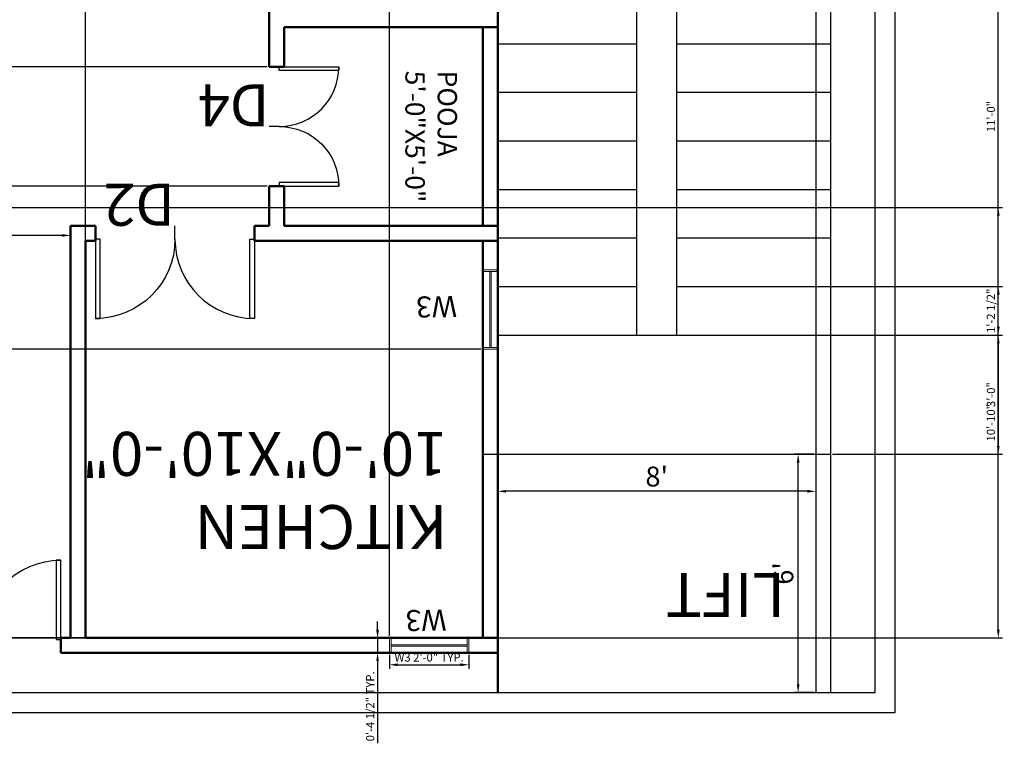
# Model space of a CAD drawing. Units: inches. Extents: x 1989 to 2637, y 1032 to 1611.
# Tile 3 of 5: x 2340 to 2637, y 1056 to 1274. Entities that reach past the tile are written whole.
import ezdxf

# ---------------------------------------------------------------- set-up
doc = ezdxf.new("R2010")
doc.units = ezdxf.units.IN
for name, color, linetype, lineweight in [('A-ANNO-TEXT', 1, 'Continuous', 18), ('A-AREA-IDEN', 1, 'Continuous', 25), ('C-PROP', 7, 'Continuous', 25), ('DIMENSIONS', 7, 'Continuous', 18), ('doors', 5, 'Continuous', 25), ('stair case', 6, 'Continuous', 25), ('walls', 7, 'Continuous', 50), ('windows', 3, 'Continuous', 18)]:
    doc.layers.add(name, color=color, linetype=linetype, lineweight=lineweight)
doc.styles.get("Standard").update_dxf_attribs({"font": 'arial.ttf'})
doc.dimstyles.new('ISO-25', dxfattribs={"dimtxt": 2.5, "dimasz": 2.5, "dimexe": 1.25, "dimexo": 0.625, "dimtad": 1, "dimlunit": 4, "dimtxsty": 'Standard', "dimcen": 2.5, "dimadec": 0, "dimazin": 0, "dimtfac": 1, "dimtmove": 0, "dimatfit": 3, "dimfxl": 1, "dimarcsym": 0})

# ---------------------------------------------------------------- blocks, each defined once
blk = doc.blocks.new('*U2')
for p, q in [((0, 0), (0, -5)), ((30, 0), (30, -5))]:
    blk.add_line(p, q)
blk.add_lwpolyline([(0, 0), (0, 30), (1.75, 30), (1.75, 0)], close=True)
blk.add_arc((0, 0), 30, 0, 90)
blk = doc.blocks.new('*D9')
at = {"layer": 'Defpoints', "color": 0, "transparency": 16777216}
for p in [(2484.5, 1142.92), (2580.5, 1142.92), (2484.5, 1131.72)]:
    blk.add_point(p, dxfattribs=at)
at = {"layer": 'DIMENSIONS', "color": 0, "lineweight": -2, "transparency": 16777216}
for p, q in [((2484.5, 1142.3), (2484.5, 1130.47)), ((2580.5, 1142.3), (2580.5, 1130.47)), ((2578, 1131.72), (2487, 1131.72))]:
    blk.add_line(p, q, dxfattribs=at)
at = {"layer": 'DIMENSIONS', "color": 0, "transparency": 16777216}
for points in [[(2487, 1132.14), (2487, 1131.31), (2484.5, 1131.72)], [(2578, 1132.14), (2578, 1131.31), (2580.5, 1131.72)]]:
    blk.add_solid(points, dxfattribs=at)
at = {"layer": 'DIMENSIONS', "color": 0, "transparency": 16777216, "insert": (2532.5, 1135.41), "char_height": 6, "attachment_point": 5}
blk.add_mtext("8'", dxfattribs=at)
blk = doc.blocks.new('*D10')
at = {"layer": 'Defpoints', "color": 0, "transparency": 16777216}
for p in [(2575.2, 1142.92), (2580.5, 1142.92), (2580.5, 1070.92)]:
    blk.add_point(p, dxfattribs=at)
at = {"layer": 'DIMENSIONS', "color": 0, "lineweight": -2, "transparency": 16777216}
for p, q in [((2579.87, 1142.92), (2573.95, 1142.92)), ((2575.2, 1073.42), (2575.2, 1140.42)), ((2579.87, 1070.92), (2573.95, 1070.92))]:
    blk.add_line(p, q, dxfattribs=at)
at = {"layer": 'DIMENSIONS', "color": 0, "transparency": 16777216}
for points in [[(2574.79, 1140.42), (2575.62, 1140.42), (2575.2, 1142.92)], [(2574.79, 1073.42), (2575.62, 1073.42), (2575.2, 1070.92)]]:
    blk.add_solid(points, dxfattribs=at)
at = {"layer": 'DIMENSIONS', "color": 0, "transparency": 16777216, "insert": (2571.51, 1106.92), "char_height": 6, "attachment_point": 5, "rotation": 90}
blk.add_mtext("6'", dxfattribs=at)
blk = doc.blocks.new('*D16')
at = {"layer": 'Defpoints', "color": 0, "transparency": 16777216}
for p in [(2259.5, 1209.01), (2259.5, 1190.91), (2355.5, 1190.91)]:
    blk.add_point(p, dxfattribs=at)
at = {"layer": 'DIMENSIONS', "color": 0, "lineweight": -2, "transparency": 16777216}
for p, q in [((2259.5, 1191.53), (2259.5, 1210.26)), ((2355.5, 1191.53), (2355.5, 1210.26)), ((2353, 1209.01), (2262, 1209.01))]:
    blk.add_line(p, q, dxfattribs=at)
at = {"layer": 'DIMENSIONS', "color": 0, "transparency": 16777216}
for points in [[(2262, 1209.43), (2262, 1208.6), (2259.5, 1209.01)], [(2353, 1209.43), (2353, 1208.6), (2355.5, 1209.01)]]:
    blk.add_solid(points, dxfattribs=at)
at = {"layer": 'DIMENSIONS', "color": 0, "transparency": 16777216, "insert": (2307.5, 1212.7), "char_height": 6, "attachment_point": 5}
blk.add_mtext("8'", dxfattribs=at)
blk = doc.blocks.new('WIN-W3-24IN')
for p, q in [((0, 0), (0, 23.95)), ((0, 23.95), (4.5, 23.95)), ((4.5, 23.95), (4.5, 0)), ((0, 23.45), (4.5, 23.45)), ((2.05, 23.45), (2.05, 0.5)), ((2.45, 23.45), (2.45, 0.5)), ((4.5, 0.5), (0, 0.5)), ((4.5, 0), (0, 0))]:
    blk.add_line(p, q)
blk = doc.blocks.new('*D24')
at = {"layer": 'Defpoints', "color": 0, "transparency": 16777216}
for p in [(2451.78, 1082.92), (2475.73, 1082.92), (2475.73, 1079.33)]:
    blk.add_point(p, dxfattribs=at)
at = {"layer": 'DIMENSIONS', "color": 0, "lineweight": -2, "transparency": 16777216}
for p, q in [((2451.78, 1082.3), (2451.78, 1078.08)), ((2475.73, 1082.3), (2475.73, 1078.08)), ((2454.28, 1079.33), (2473.23, 1079.33))]:
    blk.add_line(p, q, dxfattribs=at)
at = {"layer": 'DIMENSIONS', "color": 0, "transparency": 16777216}
for points in [[(2454.28, 1079.75), (2454.28, 1078.91), (2451.78, 1079.33)], [(2473.23, 1079.75), (2473.23, 1078.91), (2475.73, 1079.33)]]:
    blk.add_solid(points, dxfattribs=at)
at = {"layer": 'DIMENSIONS', "color": 0, "transparency": 16777216, "insert": (2463.75, 1081.23), "char_height": 2.5, "attachment_point": 5}
blk.add_mtext('W3 2\'-0" TYP.', dxfattribs=at)
blk = doc.blocks.new('*D25')
at = {"layer": 'Defpoints', "color": 0, "transparency": 16777216}
for p in [(2451.78, 1087.42), (2448.18, 1082.92), (2451.78, 1082.92)]:
    blk.add_point(p, dxfattribs=at)
at = {"layer": 'DIMENSIONS', "color": 0, "lineweight": -2, "transparency": 16777216}
for p, q in [((2448.18, 1089.92), (2448.18, 1092.42)), ((2451.15, 1087.42), (2446.93, 1087.42)), ((2448.18, 1087.42), (2448.18, 1082.92)), ((2451.15, 1082.92), (2446.93, 1082.92)), ((2448.18, 1080.42), (2448.18, 1055.61))]:
    blk.add_line(p, q, dxfattribs=at)
at = {"layer": 'DIMENSIONS', "color": 0, "transparency": 16777216}
for points in [[(2447.77, 1089.92), (2448.6, 1089.92), (2448.18, 1087.42)], [(2447.77, 1080.42), (2448.6, 1080.42), (2448.18, 1082.92)]]:
    blk.add_solid(points, dxfattribs=at)
at = {"layer": 'DIMENSIONS', "color": 0, "transparency": 16777216, "insert": (2446.27, 1066.76), "char_height": 2.5, "attachment_point": 5, "rotation": 90}
blk.add_mtext('0\'-4 1/2" TYP.', dxfattribs=at)
blk = doc.blocks.new('*D47')
at = {"layer": 'Defpoints', "color": 0, "transparency": 16777216}
for p in [(2580.5, 1310.92), (2635.65, 1310.92), (2585, 1178.92)]:
    blk.add_point(p, dxfattribs=at)
at = {"layer": 'DIMENSIONS', "color": 0, "lineweight": -2, "transparency": 16777216}
for p, q in [((2581.12, 1310.92), (2636.9, 1310.92)), ((2635.65, 1181.42), (2635.65, 1308.42)), ((2585.62, 1178.92), (2636.9, 1178.92))]:
    blk.add_line(p, q, dxfattribs=at)
at = {"layer": 'DIMENSIONS', "color": 0, "transparency": 16777216}
for points in [[(2635.23, 1308.42), (2636.06, 1308.42), (2635.65, 1310.92)], [(2635.23, 1181.42), (2636.06, 1181.42), (2635.65, 1178.92)]]:
    blk.add_solid(points, dxfattribs=at)
at = {"layer": 'DIMENSIONS', "color": 0, "transparency": 16777216, "insert": (2633.75, 1244.92), "char_height": 2.5, "attachment_point": 5, "rotation": 90}
blk.add_mtext('11\'-0"', dxfattribs=at)
blk = doc.blocks.new('*D48')
at = {"layer": 'Defpoints', "color": 0, "transparency": 16777216}
for p in [(2585, 1178.92), (2585, 1142.92), (2635.65, 1142.92)]:
    blk.add_point(p, dxfattribs=at)
at = {"layer": 'DIMENSIONS', "color": 0, "lineweight": -2, "transparency": 16777216}
for p, q in [((2585.62, 1178.92), (2636.9, 1178.92)), ((2635.65, 1176.42), (2635.65, 1145.42)), ((2585.62, 1142.92), (2636.9, 1142.92))]:
    blk.add_line(p, q, dxfattribs=at)
at = {"layer": 'DIMENSIONS', "color": 0, "transparency": 16777216}
for points in [[(2635.23, 1176.42), (2636.06, 1176.42), (2635.65, 1178.92)], [(2635.23, 1145.42), (2636.06, 1145.42), (2635.65, 1142.92)]]:
    blk.add_solid(points, dxfattribs=at)
at = {"layer": 'DIMENSIONS', "color": 0, "transparency": 16777216, "insert": (2633.75, 1160.92), "char_height": 2.5, "attachment_point": 5, "rotation": 90}
blk.add_mtext('3\'-0"', dxfattribs=at)
blk = doc.blocks.new('*D51')
at = {"layer": 'Defpoints', "color": 0, "transparency": 16777216}
for p in [(2538.5, 1193.59), (2635.65, 1193.59), (2538.5, 1178.92)]:
    blk.add_point(p, dxfattribs=at)
at = {"layer": 'DIMENSIONS', "color": 0, "lineweight": -2, "transparency": 16777216}
for p, q in [((2539.12, 1193.59), (2636.9, 1193.59)), ((2635.65, 1181.42), (2635.65, 1191.09)), ((2539.12, 1178.92), (2636.9, 1178.92))]:
    blk.add_line(p, q, dxfattribs=at)
at = {"layer": 'DIMENSIONS', "color": 0, "transparency": 16777216}
for points in [[(2635.23, 1191.09), (2636.06, 1191.09), (2635.65, 1193.59)], [(2635.23, 1181.42), (2636.06, 1181.42), (2635.65, 1178.92)]]:
    blk.add_solid(points, dxfattribs=at)
at = {"layer": 'DIMENSIONS', "color": 0, "transparency": 16777216, "insert": (2633.73, 1186.25), "char_height": 2.5, "attachment_point": 5, "rotation": 90}
blk.add_mtext('1\'-2 1/2"', dxfattribs=at)
blk = doc.blocks.new('*D59')
at = {"layer": 'Defpoints', "color": 0, "transparency": 16777216}
for p in [(2033.35, 1259.92), (2415.5, 1259.92), (2415.5, 1223.92)]:
    blk.add_point(p, dxfattribs=at)
at = {"layer": 'DIMENSIONS', "color": 0, "lineweight": -2, "transparency": 16777216}
for p, q in [((2414.87, 1259.92), (2032.1, 1259.92)), ((2033.35, 1226.42), (2033.35, 1257.42)), ((2414.87, 1223.92), (2032.1, 1223.92))]:
    blk.add_line(p, q, dxfattribs=at)
at = {"layer": 'DIMENSIONS', "color": 0, "transparency": 16777216}
for points in [[(2032.93, 1257.42), (2033.76, 1257.42), (2033.35, 1259.92)], [(2032.93, 1226.42), (2033.76, 1226.42), (2033.35, 1223.92)]]:
    blk.add_solid(points, dxfattribs=at)
at = {"layer": 'DIMENSIONS', "color": 0, "transparency": 16777216, "insert": (2031.45, 1241.92), "char_height": 2.5, "attachment_point": 5, "rotation": 90}
blk.add_mtext('3\'-0"', dxfattribs=at)
blk = doc.blocks.new('*D60')
at = {"layer": 'Defpoints', "color": 0, "transparency": 16777216}
for p in [(2451.78, 1576.07), (2360, 1087.42), (2451.78, 1087.42)]:
    blk.add_point(p, dxfattribs=at)
at = {"layer": 'DIMENSIONS', "color": 0, "lineweight": -2, "transparency": 16777216}
for p, q in [((2360, 1088.05), (2360, 1577.32)), ((2362.5, 1576.07), (2449.28, 1576.07)), ((2451.78, 1088.05), (2451.78, 1577.32))]:
    blk.add_line(p, q, dxfattribs=at)
at = {"layer": 'DIMENSIONS', "color": 0, "transparency": 16777216}
for points in [[(2362.5, 1576.49), (2362.5, 1575.65), (2360, 1576.07)], [(2449.28, 1576.49), (2449.28, 1575.65), (2451.78, 1576.07)]]:
    blk.add_solid(points, dxfattribs=at)
at = {"layer": 'DIMENSIONS', "color": 0, "transparency": 16777216, "insert": (2405.89, 1577.97), "char_height": 2.5, "attachment_point": 5}
blk.add_mtext('7\'-8"', dxfattribs=at)
blk = doc.blocks.new('*D61')
at = {"layer": 'Defpoints', "color": 0, "transparency": 16777216}
for p in [(2033.35, 1174.7), (2480, 1174.7), (2480, 1087.42)]:
    blk.add_point(p, dxfattribs=at)
at = {"layer": 'DIMENSIONS', "color": 0, "lineweight": -2, "transparency": 16777216}
for p, q in [((2479.37, 1174.7), (2032.1, 1174.7)), ((2033.35, 1089.92), (2033.35, 1172.2)), ((2479.37, 1087.42), (2032.1, 1087.42))]:
    blk.add_line(p, q, dxfattribs=at)
at = {"layer": 'DIMENSIONS', "color": 0, "transparency": 16777216}
for points in [[(2032.93, 1172.2), (2033.76, 1172.2), (2033.35, 1174.7)], [(2032.93, 1089.92), (2033.76, 1089.92), (2033.35, 1087.42)]]:
    blk.add_solid(points, dxfattribs=at)
at = {"layer": 'DIMENSIONS', "color": 0, "transparency": 16777216, "insert": (2031.43, 1131.06), "char_height": 2.5, "attachment_point": 5, "rotation": 90}
blk.add_mtext('7\'-3 1/2"', dxfattribs=at)
blk = doc.blocks.new('*D62')
at = {"layer": 'Defpoints', "color": 0, "transparency": 16777216}
for p in [(2086.98, 1217.46), (2635.65, 1217.46), (2087, 1087.42)]:
    blk.add_point(p, dxfattribs=at)
at = {"layer": 'DIMENSIONS', "color": 0, "lineweight": -2, "transparency": 16777216}
for p, q in [((2087.6, 1217.46), (2636.9, 1217.46)), ((2635.65, 1089.92), (2635.65, 1214.96)), ((2087.62, 1087.42), (2636.9, 1087.42))]:
    blk.add_line(p, q, dxfattribs=at)
at = {"layer": 'DIMENSIONS', "color": 0, "transparency": 16777216}
for points in [[(2635.23, 1214.96), (2636.06, 1214.96), (2635.65, 1217.46)], [(2635.23, 1089.92), (2636.06, 1089.92), (2635.65, 1087.42)]]:
    blk.add_solid(points, dxfattribs=at)
at = {"layer": 'DIMENSIONS', "color": 0, "transparency": 16777216, "insert": (2633.75, 1152.44), "char_height": 2.5, "attachment_point": 5, "rotation": 90}
blk.add_mtext('10\'-10"', dxfattribs=at)

msp = doc.modelspace()

# ---------------------------------------------------------------- linework, layer by layer
at = {"layer": 'C-PROP'}
for p, q in [((2604.498, 1064.921), (2604.498, 1544.921)), ((2598.498, 1070.921), (2598.498, 1538.921)), ((2070.498, 1070.921), (2598.498, 1070.921)), ((2064.498, 1064.921), (2604.498, 1064.921))]:
    msp.add_line(p, q, dxfattribs=at)
at = {"layer": 'stair case'}
for p, q in [((2484.498, 1070.921), (2484.498, 1310.921)), ((2526.498, 1178.921), (2526.498, 1310.921)), ((2538.498, 1310.921), (2538.498, 1178.921)), ((2580.498, 1310.921), (2580.498, 1070.921)), ((2584.998, 1310.921), (2584.998, 1070.921)), ((2484.498, 1266.921), (2526.498, 1266.921)), ((2538.498, 1266.921), (2584.998, 1266.921)), ((2484.498, 1252.254), (2526.498, 1252.254)), ((2538.498, 1252.254), (2584.998, 1252.254)), ((2484.498, 1237.588), (2526.498, 1237.588)), ((2538.498, 1237.588), (2584.998, 1237.588)), ((2484.498, 1222.921), (2526.498, 1222.921)), ((2538.498, 1222.921), (2584.998, 1222.921)), ((2484.498, 1208.254), (2526.498, 1208.254)), ((2538.498, 1208.254), (2584.998, 1208.254)), ((2484.498, 1193.588), (2526.498, 1193.588)), ((2538.498, 1193.588), (2584.998, 1193.588)), ((2484.498, 1178.921), (2584.998, 1178.921)), ((2479.998, 1142.921), (2584.998, 1142.921))]:
    msp.add_line(p, q, dxfattribs=at)
at = {"layer": 'walls'}
for p, q in [((2484.498, 1310.921), (2484.498, 1070.921)), ((2415.498, 1276.421), (2415.498, 1259.921)), ((2419.998, 1271.921), (2484.498, 1271.921)), ((2419.998, 1271.921), (2419.998, 1259.921)), ((2419.998, 1271.921), (2419.998, 1259.921)), ((2479.998, 1271.921), (2479.998, 1211.921)), ((2419.998, 1259.921), (2415.498, 1259.921)), ((2415.498, 1223.921), (2419.998, 1223.921)), ((2415.498, 1223.921), (2415.498, 1211.921)), ((2419.998, 1223.921), (2419.998, 1211.921)), ((2355.498, 1211.921), (2355.498, 1087.421)), ((2355.498, 1211.921), (2362.998, 1211.921)), ((2362.998, 1207.421), (2362.998, 1211.921)), ((2410.998, 1211.921), (2410.998, 1207.421)), ((2410.998, 1211.921), (2415.498, 1211.921)), ((2419.998, 1211.921), (2484.498, 1211.921)), ((2359.998, 1207.421), (2359.998, 1087.421)), ((2359.998, 1207.421), (2362.998, 1207.421)), ((2359.998, 1207.421), (2362.998, 1207.421)), ((2359.998, 1207.421), (2362.998, 1207.421)), ((2410.998, 1207.421), (2484.498, 1207.421)), ((2479.998, 1207.421), (2479.998, 1087.421)), ((2355.498, 1087.421), (2352.498, 1087.421)), ((2352.498, 1087.421), (2352.498, 1082.921)), ((2352.498, 1087.421), (2355.498, 1087.421)), ((2359.998, 1087.421), (2484.498, 1087.421)), ((2352.498, 1082.921), (2484.498, 1082.921))]:
    msp.add_line(p, q, dxfattribs=at)

# ---------------------------------------------------------------- block references
at = {"layer": 'doors'}
for p, xscale, yscale, zscale, rotation in [((2418.498, 1259.921), 0.6000000000000001, 0.6000000000000001, 0.6000000000000001, 270), ((2418.498, 1223.921), -0.6000000000000001, 0.6000000000000001, 0.6000000000000001, 270), ((2362.998, 1207.921), -0.8, 0.8, 0.8, 180), ((2410.998, 1207.921), 0.8, 0.8, 0.8, 180)]:
    msp.add_blockref('*U2', p, dxfattribs=dict(at, xscale=xscale, yscale=yscale, zscale=zscale, rotation=rotation))
at = {"layer": 'doors', "xscale": -0.8, "yscale": 0.8, "zscale": 0.8}
msp.add_blockref('*U2', (2352.498, 1086.921), dxfattribs=at)
at = {"layer": 'windows'}
msp.add_blockref('WIN-W3-24IN', (2479.998, 1174.701), dxfattribs=at)
at = {"layer": 'windows', "rotation": 269.9999999999951}
msp.add_blockref('WIN-W3-24IN', (2451.776, 1087.421), dxfattribs=at)

# ---------------------------------------------------------------- texts
at = {"layer": 'A-ANNO-TEXT', "attachment_point": 1}
for s, width, gutter_width, insert, char_height, rotation in [('D4', 3.801, 63.542, (2415.498, 1241.921), 12.7085, 180), ('D2', 3.801, 63.542, (2386.998, 1211.921), 12.7085, 180), ('W3', 5.29651, 31.753, (2472.21, 1184.348), 6.3507, 180.67334), ('W3', 5.29651, 31.753, (2469.039, 1089.637), 6.3507, 180.67334)]:
    msp.add_mtext_dynamic_manual_height_columns(s, width=width, gutter_width=gutter_width, heights=[0], dxfattribs=dict(at, insert=insert, char_height=char_height, rotation=rotation))
at = {"layer": 'A-AREA-IDEN', "attachment_point": 1}
for s, width, gutter_width, insert, char_height, rotation in [('POOJA\\P5\'-0"X5\'-0"', 1.53563, 29.224, (2472.186, 1258.774), 5.84487, 270), ('KITCHEN\\P10\'-0"X10\'-0"', 13.72319, 66.348, (2469.27, 1114.28), 13.26964, 180), ('LIFT', 13.72319, 66.348, (2571.227, 1093.803), 13.2696, 180)]:
    msp.add_mtext_dynamic_manual_height_columns(s, width=width, gutter_width=gutter_width, heights=[0], dxfattribs=dict(at, insert=insert, char_height=char_height, rotation=rotation))

# ---------------------------------------------------------------- dimensions: what is measured, and where the dimension line sits
at = {"layer": 'DIMENSIONS'}
for base, p1, p2, override, picture, middle in [((2451.776, 1576.071), (2359.998, 1087.421), (2451.776, 1087.421), {"dimdec": 1, "dimlfac": 1, "dimrnd": 0, "dimzin": 1, "dimdsep": 46, "dimlunit": 4, "dimfrac": 2}, '*D60', (2405.887, 1577.972)), ((2259.498, 1209.015), (2355.498, 1190.907), (2259.498, 1190.907), {"dimtxt": 6, "dimclrd": 0, "dimclre": 0, "dimclrt": 0}, '*D16', (2307.498, 1212.703)), ((2484.498, 1131.722), (2580.498, 1142.921), (2484.498, 1142.921), {"dimtxt": 6, "dimclrd": 0, "dimclre": 0, "dimclrt": 0}, '*D9', (2532.498, 1135.411))]:
    dim = msp.add_linear_dim(base=base, p1=p1, p2=p2, dimstyle='ISO-25', override=override, dxfattribs=at)
    dim.commit()
    dim.dimension.update_dxf_attribs({"geometry": picture, "text_midpoint": middle})
for base, p1, p2, override, picture, middle in [((2635.648, 1310.921), (2584.998, 1178.921), (2580.498, 1310.921), {"dimdec": 1, "dimlfac": 1, "dimrnd": 0, "dimzin": 1, "dimdsep": 46, "dimlunit": 4, "dimfrac": 2}, '*D47', (2633.746, 1244.921)), ((2033.348, 1259.921), (2415.498, 1223.921), (2415.498, 1259.921), {"dimdec": 1, "dimlfac": 1, "dimrnd": 0, "dimzin": 1, "dimdsep": 46, "dimlunit": 4, "dimfrac": 2}, '*D59', (2031.445, 1241.921)), ((2635.648, 1217.461), (2086.998, 1087.421), (2086.98, 1217.461), {"dimdec": 1, "dimlfac": 1, "dimrnd": 0, "dimzin": 1, "dimdsep": 46, "dimlunit": 4, "dimfrac": 2}, '*D62', (2633.746, 1152.441)), ((2635.648, 1193.588), (2538.498, 1178.921), (2538.498, 1193.588), {"dimdec": 1, "dimlfac": 1, "dimrnd": 0, "dimzin": 1, "dimdsep": 46, "dimlunit": 4, "dimfrac": 2}, '*D51', (2633.73, 1186.254)), ((2635.648, 1142.921), (2584.998, 1178.921), (2584.998, 1142.921), {"dimdec": 1, "dimlfac": 1, "dimrnd": 0, "dimzin": 1, "dimdsep": 46, "dimlunit": 4, "dimfrac": 2}, '*D48', (2633.745, 1160.921)), ((2033.348, 1174.701), (2479.998, 1087.421), (2479.998, 1174.701), {"dimdec": 1, "dimlfac": 1, "dimrnd": 0, "dimzin": 1, "dimdsep": 46, "dimlunit": 4, "dimfrac": 2}, '*D61', (2031.429, 1131.061)), ((2575.202, 1142.921), (2580.498, 1070.921), (2580.498, 1142.921), {"dimtxt": 6, "dimclrd": 0, "dimclre": 0, "dimclrt": 0}, '*D10', (2571.514, 1106.921))]:
    dim = msp.add_linear_dim(base=base, p1=p1, p2=p2, angle=90, dimstyle='ISO-25', override=override, dxfattribs=at)
    dim.commit()
    dim.dimension.update_dxf_attribs({"geometry": picture, "text_midpoint": middle})
dim = msp.add_linear_dim(base=(2448.184, 1082.921), p1=(2451.776, 1087.421), p2=(2451.776, 1082.921), angle=270, text='<> TYP.', dimstyle='ISO-25', override={"dimdec": 1, "dimlfac": 1, "dimrnd": 0, "dimzin": 1, "dimdsep": 46, "dimlunit": 4, "dimfrac": 2}, dxfattribs=at)
dim.commit()
dim.dimension.update_dxf_attribs({"geometry": '*D25', "text_midpoint": (2446.266, 1066.764)})
dim = msp.add_linear_dim(base=(2475.7261, 1079.3284), p1=(2451.7764, 1082.9209), p2=(2475.7261, 1082.9209), text='W3 <> TYP.', dimstyle='ISO-25', override={"dimdec": 1, "dimlfac": 1, "dimrnd": 0, "dimzin": 1, "dimdsep": 46, "dimlunit": 4, "dimfrac": 2}, dxfattribs=at)
dim.commit()
dim.dimension.update_dxf_attribs({"geometry": '*D24', "text_midpoint": (2463.7512, 1081.2307)})

doc.saveas('drawing.dxf')
